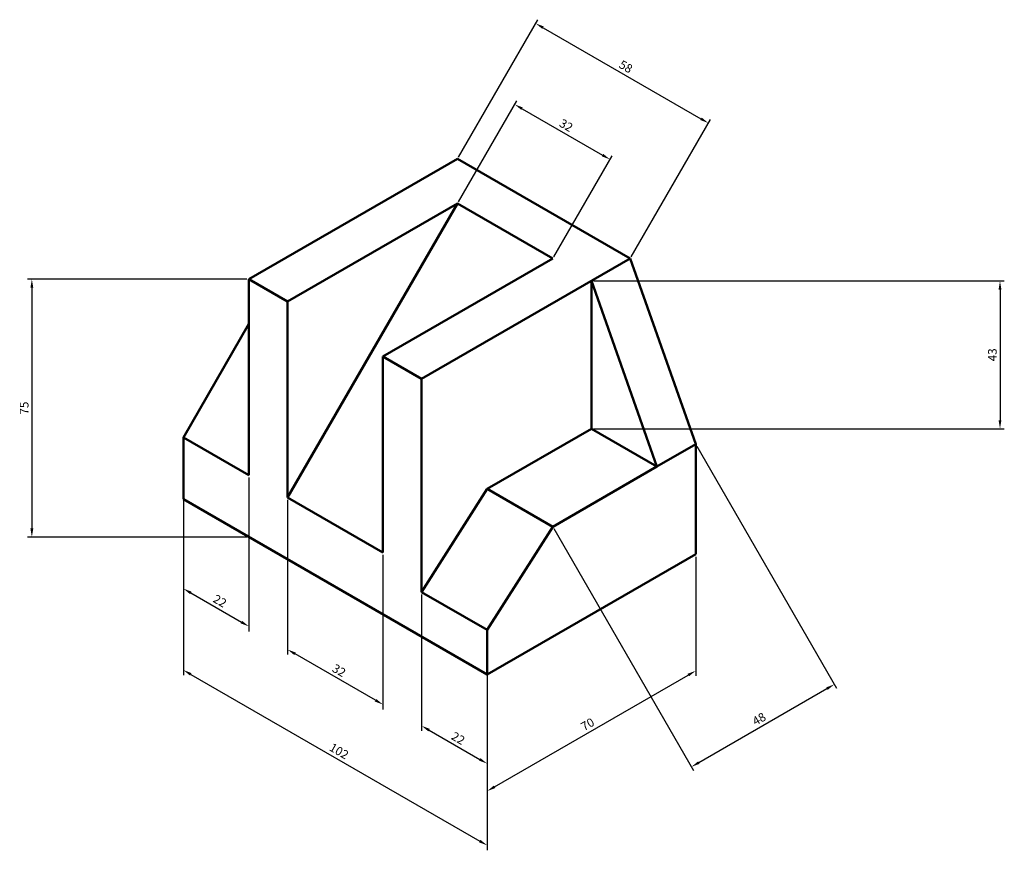
# Model space of a CAD drawing. Units: millimetres. Extents: x 5229 to 5516, y 2960 to 3202.
import ezdxf

# ---------------------------------------------------------------- set-up
doc = ezdxf.new("R2010")
doc.units = ezdxf.units.MM
doc.layers.add('M-DIMS', color=2, linetype='Continuous', lineweight=25)
doc.layers.add('M-OUTL', color=7, linetype='Continuous', lineweight=50)
doc.styles.get("Standard").update_dxf_attribs({"font": 'arial.ttf'})
doc.dimstyles.new('ISO-25', dxfattribs={"dimtxt": 2.5, "dimasz": 2.5, "dimexe": 1.25, "dimexo": 0.625, "dimtad": 1, "dimtxsty": 'Standard', "dimcen": 2.5, "dimadec": 0, "dimazin": 0, "dimtfac": 1, "dimtmove": 0, "dimatfit": 3, "dimfxl": 1, "dimarcsym": 0})

# ---------------------------------------------------------------- blocks, each defined once
blk = doc.blocks.new('*D1')
at = {"layer": 'Defpoints', "color": 0, "transparency": 16777216}
for p in [(5425.89, 3046.57), (5365.27, 3011.57), (5425.89, 3012.67)]:
    blk.add_point(p, dxfattribs=at)
at = {"layer": 'M-DIMS', "color": 0, "lineweight": -2, "transparency": 16777216}
for p, q in [((5425.89, 3045.85), (5425.89, 3011.23)), ((5365.27, 3010.85), (5365.27, 2976.23)), ((5367.43, 2978.92), (5423.72, 3011.42))]:
    blk.add_line(p, q, dxfattribs=at)
at = {"layer": 'M-DIMS', "color": 0, "transparency": 16777216}
for points in [[(5423.52, 3011.78), (5423.93, 3011.06), (5425.89, 3012.67)], [(5367.22, 2979.28), (5367.64, 2978.56), (5365.27, 2977.67)]]:
    blk.add_solid(points, dxfattribs=at)
at = {"layer": 'M-DIMS', "color": 0, "transparency": 16777216, "insert": (5394.63, 2996.82), "char_height": 2.5, "attachment_point": 5, "rotation": 30}
blk.add_mtext('70', dxfattribs=at)
blk = doc.blocks.new('*D2')
at = {"layer": 'Defpoints', "color": 0, "transparency": 16777216}
for p in [(5276.93, 3062.57), (5365.27, 3011.57), (5365.27, 2961.88)]:
    blk.add_point(p, dxfattribs=at)
at = {"layer": 'M-DIMS', "color": 0, "lineweight": -2, "transparency": 16777216}
for p, q in [((5276.93, 3061.85), (5276.93, 3011.44)), ((5279.1, 3011.63), (5363.1, 2963.13)), ((5365.27, 3010.85), (5365.27, 2960.44))]:
    blk.add_line(p, q, dxfattribs=at)
at = {"layer": 'M-DIMS', "color": 0, "transparency": 16777216}
for points in [[(5279.31, 3011.99), (5278.89, 3011.27), (5276.93, 3012.88)], [(5363.31, 2963.49), (5362.89, 2962.77), (5365.27, 2961.88)]]:
    blk.add_solid(points, dxfattribs=at)
at = {"layer": 'M-DIMS', "color": 0, "transparency": 16777216, "insert": (5322.05, 2989.03), "char_height": 2.5, "attachment_point": 5, "rotation": 330}
blk.add_mtext('102', dxfattribs=at)
blk = doc.blocks.new('*D3')
at = {"layer": 'Defpoints', "color": 0, "transparency": 16777216}
for p in [(5346.21, 3035.57), (5365.27, 3024.57), (5365.27, 2985.65)]:
    blk.add_point(p, dxfattribs=at)
at = {"layer": 'M-DIMS', "color": 0, "lineweight": -2, "transparency": 16777216}
for p, q in [((5346.21, 3034.85), (5346.21, 2995.2)), ((5365.27, 3023.85), (5365.27, 2984.2)), ((5348.38, 2995.4), (5363.1, 2986.9))]:
    blk.add_line(p, q, dxfattribs=at)
at = {"layer": 'M-DIMS', "color": 0, "transparency": 16777216}
for points in [[(5348.59, 2995.76), (5348.17, 2995.04), (5346.21, 2996.65)], [(5363.31, 2987.26), (5362.89, 2986.54), (5365.27, 2985.65)]]:
    blk.add_solid(points, dxfattribs=at)
at = {"layer": 'M-DIMS', "color": 0, "transparency": 16777216, "insert": (5356.68, 2992.77), "char_height": 2.5, "attachment_point": 5, "rotation": 330}
blk.add_mtext('22', dxfattribs=at)
blk = doc.blocks.new('*D4')
at = {"layer": 'Defpoints', "color": 0, "transparency": 16777216}
for p in [(5307.24, 3063.07), (5334.96, 3047.07), (5307.24, 3018.85)]:
    blk.add_point(p, dxfattribs=at)
at = {"layer": 'M-DIMS', "color": 0, "lineweight": -2, "transparency": 16777216}
for p, q in [((5307.24, 3062.35), (5307.24, 3017.4)), ((5334.96, 3046.35), (5334.96, 3001.4)), ((5332.79, 3004.1), (5309.41, 3017.6))]:
    blk.add_line(p, q, dxfattribs=at)
at = {"layer": 'M-DIMS', "color": 0, "transparency": 16777216}
for points in [[(5309.62, 3017.96), (5309.2, 3017.23), (5307.24, 3018.85)], [(5333, 3004.46), (5332.58, 3003.73), (5334.96, 3002.85)]]:
    blk.add_solid(points, dxfattribs=at)
at = {"layer": 'M-DIMS', "color": 0, "transparency": 16777216, "insert": (5322.05, 3012.49), "char_height": 2.5, "attachment_point": 5, "rotation": 330}
blk.add_mtext('32', dxfattribs=at)
blk = doc.blocks.new('*D5')
at = {"layer": 'Defpoints', "color": 0, "transparency": 16777216}
for p in [(5276.93, 3080.57), (5295.99, 3069.57), (5295.99, 3025.57)]:
    blk.add_point(p, dxfattribs=at)
at = {"layer": 'M-DIMS', "color": 0, "lineweight": -2, "transparency": 16777216}
for p, q in [((5276.93, 3079.85), (5276.93, 3035.13)), ((5295.99, 3068.85), (5295.99, 3024.13)), ((5279.1, 3035.32), (5293.82, 3026.82))]:
    blk.add_line(p, q, dxfattribs=at)
at = {"layer": 'M-DIMS', "color": 0, "transparency": 16777216}
for points in [[(5279.31, 3035.68), (5278.89, 3034.96), (5276.93, 3036.57)], [(5294.03, 3027.18), (5293.61, 3026.46), (5295.99, 3025.57)]]:
    blk.add_solid(points, dxfattribs=at)
at = {"layer": 'M-DIMS', "color": 0, "transparency": 16777216, "insert": (5287.4, 3032.7), "char_height": 2.5, "attachment_point": 5, "rotation": 330}
blk.add_mtext('22', dxfattribs=at)
blk = doc.blocks.new('*D6')
at = {"layer": 'Defpoints', "color": 0, "transparency": 16777216}
for p in [(5295.99, 3126.57), (5232.89, 3051.57), (5295.99, 3051.57)]:
    blk.add_point(p, dxfattribs=at)
at = {"layer": 'M-DIMS', "color": 0, "lineweight": -2, "transparency": 16777216}
for p, q in [((5295.36, 3126.57), (5231.64, 3126.57)), ((5232.89, 3124.07), (5232.89, 3054.07)), ((5295.36, 3051.57), (5231.64, 3051.57))]:
    blk.add_line(p, q, dxfattribs=at)
at = {"layer": 'M-DIMS', "color": 0, "transparency": 16777216}
for points in [[(5232.47, 3124.07), (5233.31, 3124.07), (5232.89, 3126.57)], [(5232.47, 3054.07), (5233.31, 3054.07), (5232.89, 3051.57)]]:
    blk.add_solid(points, dxfattribs=at)
at = {"layer": 'M-DIMS', "color": 0, "transparency": 16777216, "insert": (5230.99, 3089.07), "char_height": 2.5, "attachment_point": 5, "rotation": 90}
blk.add_mtext('75', dxfattribs=at)
blk = doc.blocks.new('*D7')
at = {"layer": 'Defpoints', "color": 0, "transparency": 16777216}
for p in [(5400.97, 3161.42), (5356.61, 3148.57), (5384.32, 3132.57)]:
    blk.add_point(p, dxfattribs=at)
at = {"layer": 'M-DIMS', "color": 0, "lineweight": -2, "transparency": 16777216}
for p, q in [((5356.92, 3149.12), (5373.89, 3178.5)), ((5375.43, 3176.17), (5398.81, 3162.67)), ((5384.63, 3133.12), (5401.6, 3162.5))]:
    blk.add_line(p, q, dxfattribs=at)
at = {"layer": 'M-DIMS', "color": 0, "transparency": 16777216}
for points in [[(5375.63, 3176.53), (5375.22, 3175.81), (5373.26, 3177.42)], [(5399.02, 3163.03), (5398.6, 3162.31), (5400.97, 3161.42)]]:
    blk.add_solid(points, dxfattribs=at)
at = {"layer": 'M-DIMS', "color": 0, "transparency": 16777216, "insert": (5388.07, 3171.07), "char_height": 2.5, "attachment_point": 5, "rotation": 330}
blk.add_mtext('32', dxfattribs=at)
blk = doc.blocks.new('*D8')
at = {"layer": 'Defpoints', "color": 0, "transparency": 16777216}
for p in [(5429.59, 3171.99), (5356.61, 3161.57), (5406.84, 3132.57)]:
    blk.add_point(p, dxfattribs=at)
at = {"layer": 'M-DIMS', "color": 0, "lineweight": -2, "transparency": 16777216}
for p, q in [((5356.92, 3162.12), (5379.99, 3202.07)), ((5381.53, 3199.74), (5427.43, 3173.24)), ((5407.15, 3133.12), (5430.22, 3173.07))]:
    blk.add_line(p, q, dxfattribs=at)
at = {"layer": 'M-DIMS', "color": 0, "transparency": 16777216}
for points in [[(5381.74, 3200.1), (5381.32, 3199.38), (5379.36, 3200.99)], [(5427.64, 3173.6), (5427.22, 3172.88), (5429.59, 3171.99)]]:
    blk.add_solid(points, dxfattribs=at)
at = {"layer": 'M-DIMS', "color": 0, "transparency": 16777216, "insert": (5405.43, 3188.14), "char_height": 2.5, "attachment_point": 5, "rotation": 330}
blk.add_mtext('58', dxfattribs=at)
blk = doc.blocks.new('*D9')
at = {"layer": 'Defpoints', "color": 0, "transparency": 16777216}
for p in [(5395.58, 3126.07), (5395.58, 3083.07), (5514.37, 3083.07)]:
    blk.add_point(p, dxfattribs=at)
at = {"layer": 'M-DIMS', "color": 0, "lineweight": -2, "transparency": 16777216}
for p, q in [((5396.2, 3126.07), (5515.62, 3126.07)), ((5514.37, 3123.57), (5514.37, 3085.57)), ((5396.2, 3083.07), (5515.62, 3083.07))]:
    blk.add_line(p, q, dxfattribs=at)
at = {"layer": 'M-DIMS', "color": 0, "transparency": 16777216}
for points in [[(5513.95, 3123.57), (5514.78, 3123.57), (5514.37, 3126.07)], [(5513.95, 3085.57), (5514.78, 3085.57), (5514.37, 3083.07)]]:
    blk.add_solid(points, dxfattribs=at)
at = {"layer": 'M-DIMS', "color": 0, "transparency": 16777216, "insert": (5512.47, 3104.57), "char_height": 2.5, "attachment_point": 5, "rotation": 90}
blk.add_mtext('43', dxfattribs=at)
blk = doc.blocks.new('*D10')
at = {"layer": 'Defpoints', "color": 0, "transparency": 16777216}
for p in [(5425.89, 3078.57), (5384.32, 3054.57), (5466.22, 3008.72)]:
    blk.add_point(p, dxfattribs=at)
at = {"layer": 'M-DIMS', "color": 0, "lineweight": -2, "transparency": 16777216}
for p, q in [((5426.2, 3078.03), (5466.85, 3007.64)), ((5384.63, 3054.03), (5425.28, 2983.64)), ((5426.82, 2985.97), (5464.05, 3007.47))]:
    blk.add_line(p, q, dxfattribs=at)
at = {"layer": 'M-DIMS', "color": 0, "transparency": 16777216}
for points in [[(5463.85, 3007.83), (5464.26, 3007.11), (5466.22, 3008.72)], [(5426.61, 2986.33), (5427.02, 2985.61), (5424.65, 2984.72)]]:
    blk.add_solid(points, dxfattribs=at)
at = {"layer": 'M-DIMS', "color": 0, "transparency": 16777216, "insert": (5444.48, 2998.37), "char_height": 2.5, "attachment_point": 5, "rotation": 30}
blk.add_mtext('48', dxfattribs=at)

msp = doc.modelspace()

# ---------------------------------------------------------------- linework, layer by layer
at = {"layer": 'M-OUTL'}
for p, q in [((5295.985, 3126.574), (5356.607, 3161.574)), ((5356.607, 3161.574), (5406.836, 3132.574)), ((5356.607, 3148.574), (5307.244, 3120.074)), ((5307.244, 3063.074), (5356.607, 3148.574)), ((5384.32, 3132.574), (5356.607, 3148.574)), ((5334.956, 3104.074), (5384.32, 3132.574)), ((5346.215, 3097.574), (5406.836, 3132.574)), ((5406.836, 3132.574), (5425.889, 3078.574)), ((5307.244, 3120.074), (5295.985, 3126.574)), ((5295.985, 3126.574), (5295.985, 3069.574)), ((5395.578, 3126.074), (5414.631, 3072.074)), ((5395.578, 3126.074), (5395.578, 3083.074)), ((5307.244, 3063.074), (5307.244, 3120.074)), ((5276.933, 3080.574), (5295.985, 3113.574)), ((5346.215, 3097.574), (5334.956, 3104.074)), ((5334.956, 3104.074), (5334.956, 3047.074)), ((5346.215, 3035.574), (5346.215, 3097.574)), ((5295.985, 3069.574), (5276.933, 3080.574)), ((5276.933, 3080.574), (5276.933, 3062.574)), ((5365.267, 3065.574), (5395.578, 3083.074)), ((5395.578, 3083.074), (5414.631, 3072.074)), ((5425.889, 3078.574), (5414.631, 3072.074)), ((5425.889, 3046.574), (5425.889, 3078.574)), ((5414.631, 3072.074), (5384.32, 3054.574)), ((5334.956, 3047.074), (5307.244, 3063.074)), ((5346.215, 3035.574), (5365.267, 3065.574)), ((5384.32, 3054.574), (5365.267, 3065.574)), ((5276.933, 3062.574), (5365.267, 3011.574)), ((5365.267, 3024.574), (5384.32, 3054.574)), ((5365.267, 3011.574), (5425.889, 3046.574)), ((5365.267, 3024.574), (5346.215, 3035.574)), ((5365.267, 3011.574), (5365.267, 3024.574))]:
    msp.add_line(p, q, dxfattribs=at)

# ---------------------------------------------------------------- dimensions: what is measured, and where the dimension line sits
at = {"layer": 'M-DIMS'}
for p1, p2, distance, picture, middle in [((5356.607, 3161.574), (5406.836, 3132.574), 45.513, '*D8', (5405.429, 3188.136)), ((5356.607, 3148.574), (5384.32, 3132.574), 33.307, '*D7', (5388.068, 3171.066)), ((5295.985, 3126.574), (5295.985, 3051.574), -63.097, '*D6', (5230.992, 3089.074)), ((5395.578, 3126.074), (5395.578, 3083.074), 118.79, '*D9', (5512.466, 3104.574)), ((5276.933, 3080.574), (5295.985, 3069.574), -38.105, '*D5', (5287.399, 3032.702)), ((5384.32, 3054.574), (5425.889, 3078.574), -80.662, '*D10', (5444.485, 2998.365)), ((5334.956, 3047.074), (5307.244, 3063.074), 38.303, '*D4', (5322.051, 3012.493)), ((5276.933, 3062.574), (5365.267, 3011.574), -43.033, '*D2', (5322.051, 2989.03)), ((5365.267, 3011.574), (5425.889, 3046.574), -29.359, '*D1', (5394.627, 2996.82)), ((5346.215, 3035.574), (5365.267, 3024.574), -33.712, '*D3', (5356.681, 2992.774))]:
    dim = msp.add_aligned_dim(p1=p1, p2=p2, distance=distance, dimstyle='ISO-25', override={"dimclrd": 0, "dimclre": 0, "dimclrt": 0}, dxfattribs=at)
    dim.commit()
    dim.dimension.update_dxf_attribs({"geometry": picture, "text_midpoint": middle})

doc.saveas('drawing.dxf')
